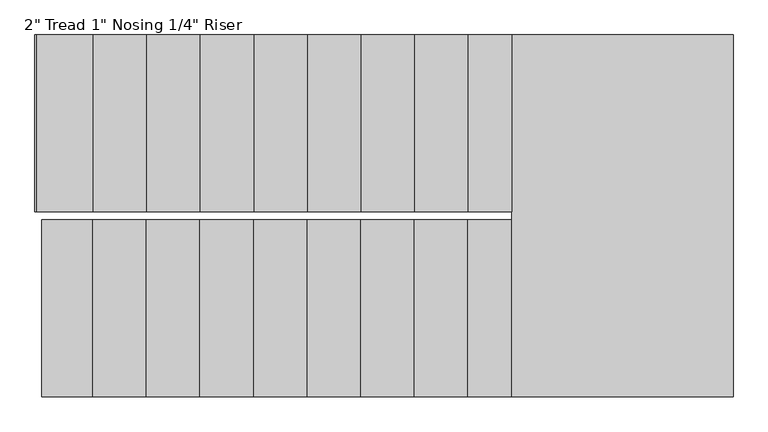
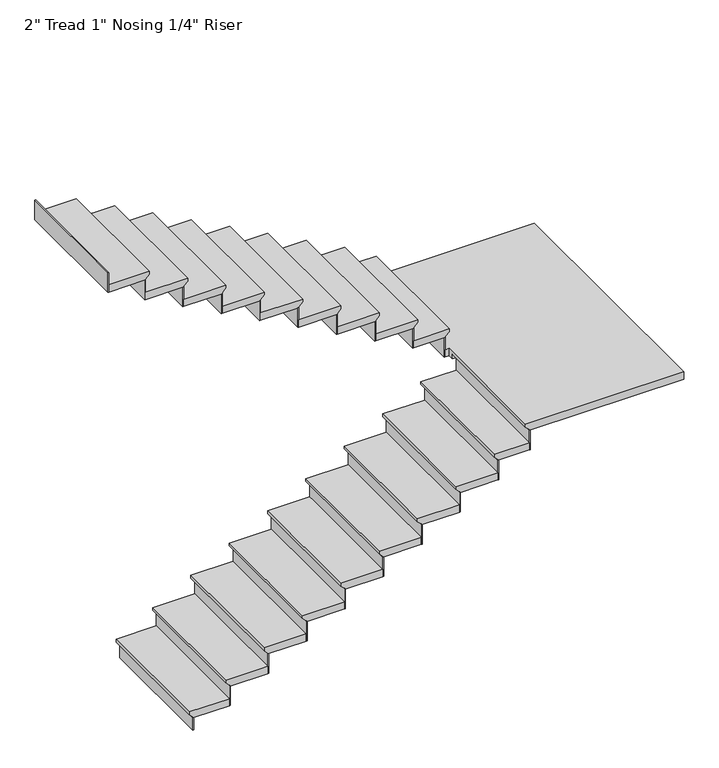
"""IFC4 building model written with IfcOpenShell, lengths in millimetres: stair flight geometry."""

from ifc_helpers import new_model, si_unit, origin, place, context, project, spatial, faceted_brep, source, transform, mapped, element, save


def stair_flight_f099b86a(model_context):
    return source(origin(), model_context, "Body", "Brep", [
        faceted_brep([(-1903.1876145, -1606.0595056, 9262.11), (-1903.1876145, -1606.0595056, 9281.16), (-1903.1876145, -767.8595056, 9281.16), (-1903.1876145, -767.8595056, 9262.11), (-1877.7876145, -1606.0595056, 9236.71), (-1877.7876145, -767.8595056, 9236.71), (-1635.543606, -1606.0595056, 9281.16), (-1635.543606, -767.8595056, 9281.16), (-1877.7876145, -767.8595056, 9230.36), (-1635.543606, -767.8595056, 9230.36), (-1635.543606, -1606.0595056, 9230.36), (-1877.7876145, -1606.0595056, 9230.36)], [[[0, 1, 2, 3]], [[4, 0, 3, 5]], [[2, 1, 6, 7]], [[8, 9, 10, 11]], [[2, 7, 9, 8, 5, 3]], [[8, 11, 4, 5]], [[6, 1, 0, 4, 11, 10]], [[7, 6, 10, 9]]]),
        faceted_brep([(-1877.7876145, -1606.0595056, 9230.36), (-1877.7876145, -1606.0595056, 9144.0), (-1871.4376145, -1606.0595056, 9144.0), (-1871.4376145, -1606.0595056, 9230.36), (-1877.7876145, -767.8595056, 9230.36), (-1871.4376145, -767.8595056, 9230.36), (-1871.4376145, -767.8595056, 9144.0), (-1877.7876145, -767.8595056, 9144.0)], [[[0, 1, 2, 3]], [[4, 5, 6, 7]], [[1, 0, 4, 7]], [[2, 1, 7, 6]], [[3, 2, 6, 5]], [[0, 3, 5, 4]]]),
        faceted_brep([(-1635.543606, -1606.0595056, 9367.52), (-1635.543606, -1606.0595056, 9230.36), (-1629.193606, -1606.0595056, 9230.36), (-1629.193606, -1606.0595056, 9367.52), (-1635.543606, -767.8595056, 9367.52), (-1629.193606, -767.8595056, 9367.52), (-1629.193606, -767.8595056, 9230.36), (-1635.543606, -767.8595056, 9230.36)], [[[0, 1, 2, 3]], [[4, 5, 6, 7]], [[1, 0, 4, 7]], [[2, 1, 7, 6]], [[3, 2, 6, 5]], [[0, 3, 5, 4]]]),
        faceted_brep([(-1660.943606, -767.8595056, 9418.32), (-1660.943606, -1606.0595056, 9418.32), (-1381.543606, -1606.0595056, 9418.32), (-1381.543606, -767.8595056, 9418.32), (-1635.543606, -767.8595056, 9367.52), (-1381.543606, -767.8595056, 9367.52), (-1381.543606, -1606.0595056, 9367.52), (-1635.543606, -1606.0595056, 9367.52), (-1635.543606, -767.8595056, 9373.87), (-1660.943606, -767.8595056, 9399.27), (-1635.543606, -1606.0595056, 9373.87), (-1660.943606, -1606.0595056, 9399.27)], [[[0, 1, 2, 3]], [[4, 5, 6, 7]], [[0, 3, 5, 4, 8, 9]], [[4, 7, 10, 8]], [[2, 1, 11, 10, 7, 6]], [[3, 2, 6, 5]], [[11, 1, 0, 9]], [[10, 11, 9, 8]]]),
        faceted_brep([(-1381.543606, -1606.0595056, 9504.68), (-1381.543606, -1606.0595056, 9367.52), (-1375.193606, -1606.0595056, 9367.52), (-1375.193606, -1606.0595056, 9504.68), (-1381.543606, -767.8595056, 9504.68), (-1375.193606, -767.8595056, 9504.68), (-1375.193606, -767.8595056, 9367.52), (-1381.543606, -767.8595056, 9367.52)], [[[0, 1, 2, 3]], [[4, 5, 6, 7]], [[1, 0, 4, 7]], [[2, 1, 7, 6]], [[3, 2, 6, 5]], [[0, 3, 5, 4]]]),
        faceted_brep([(-1406.943606, -767.8595056, 9555.48), (-1406.943606, -1606.0595056, 9555.48), (-1127.543606, -1606.0595056, 9555.48), (-1127.543606, -767.8595056, 9555.48), (-1381.543606, -767.8595056, 9504.68), (-1127.543606, -767.8595056, 9504.68), (-1127.543606, -1606.0595056, 9504.68), (-1381.543606, -1606.0595056, 9504.68), (-1381.543606, -767.8595056, 9511.03), (-1406.943606, -767.8595056, 9536.43), (-1381.543606, -1606.0595056, 9511.03), (-1406.943606, -1606.0595056, 9536.43)], [[[0, 1, 2, 3]], [[4, 5, 6, 7]], [[0, 3, 5, 4, 8, 9]], [[4, 7, 10, 8]], [[2, 1, 11, 10, 7, 6]], [[3, 2, 6, 5]], [[11, 1, 0, 9]], [[10, 11, 9, 8]]]),
        faceted_brep([(-1127.543606, -1606.0595056, 9641.84), (-1127.543606, -1606.0595056, 9504.68), (-1121.193606, -1606.0595056, 9504.68), (-1121.193606, -1606.0595056, 9641.84), (-1127.543606, -767.8595056, 9641.84), (-1121.193606, -767.8595056, 9641.84), (-1121.193606, -767.8595056, 9504.68), (-1127.543606, -767.8595056, 9504.68)], [[[0, 1, 2, 3]], [[4, 5, 6, 7]], [[1, 0, 4, 7]], [[2, 1, 7, 6]], [[3, 2, 6, 5]], [[0, 3, 5, 4]]]),
        faceted_brep([(-1152.943606, -767.8595056, 9692.64), (-1152.943606, -1606.0595056, 9692.64), (-873.543606, -1606.0595056, 9692.64), (-873.543606, -767.8595056, 9692.64), (-1127.543606, -767.8595056, 9641.84), (-873.543606, -767.8595056, 9641.84), (-873.543606, -1606.0595056, 9641.84), (-1127.543606, -1606.0595056, 9641.84), (-1127.543606, -767.8595056, 9648.19), (-1152.943606, -767.8595056, 9673.59), (-1127.543606, -1606.0595056, 9648.19), (-1152.943606, -1606.0595056, 9673.59)], [[[0, 1, 2, 3]], [[4, 5, 6, 7]], [[0, 3, 5, 4, 8, 9]], [[4, 7, 10, 8]], [[2, 1, 11, 10, 7, 6]], [[3, 2, 6, 5]], [[11, 1, 0, 9]], [[10, 11, 9, 8]]]),
        faceted_brep([(-873.543606, -1606.0595056, 9779.0), (-873.543606, -1606.0595056, 9641.84), (-867.193606, -1606.0595056, 9641.84), (-867.193606, -1606.0595056, 9779.0), (-873.543606, -767.8595056, 9779.0), (-867.193606, -767.8595056, 9779.0), (-867.193606, -767.8595056, 9641.84), (-873.543606, -767.8595056, 9641.84)], [[[0, 1, 2, 3]], [[4, 5, 6, 7]], [[1, 0, 4, 7]], [[2, 1, 7, 6]], [[3, 2, 6, 5]], [[0, 3, 5, 4]]]),
        faceted_brep([(-898.943606, -767.8595056, 9829.8), (-898.943606, -1606.0595056, 9829.8), (-619.543606, -1606.0595056, 9829.8), (-619.543606, -767.8595056, 9829.8), (-873.543606, -767.8595056, 9779.0), (-619.543606, -767.8595056, 9779.0), (-619.543606, -1606.0595056, 9779.0), (-873.543606, -1606.0595056, 9779.0), (-873.543606, -767.8595056, 9785.35), (-898.943606, -767.8595056, 9810.75), (-873.543606, -1606.0595056, 9785.35), (-898.943606, -1606.0595056, 9810.75)], [[[0, 1, 2, 3]], [[4, 5, 6, 7]], [[0, 3, 5, 4, 8, 9]], [[4, 7, 10, 8]], [[2, 1, 11, 10, 7, 6]], [[3, 2, 6, 5]], [[11, 1, 0, 9]], [[10, 11, 9, 8]]]),
        faceted_brep([(-619.543606, -1606.0595056, 9916.16), (-619.543606, -1606.0595056, 9779.0), (-613.193606, -1606.0595056, 9779.0), (-613.193606, -1606.0595056, 9916.16), (-619.543606, -767.8595056, 9916.16), (-613.193606, -767.8595056, 9916.16), (-613.193606, -767.8595056, 9779.0), (-619.543606, -767.8595056, 9779.0)], [[[0, 1, 2, 3]], [[4, 5, 6, 7]], [[1, 0, 4, 7]], [[2, 1, 7, 6]], [[3, 2, 6, 5]], [[0, 3, 5, 4]]]),
        faceted_brep([(-644.943606, -767.8595056, 9966.96), (-644.943606, -1606.0595056, 9966.96), (-365.543606, -1606.0595056, 9966.96), (-365.543606, -767.8595056, 9966.96), (-619.543606, -767.8595056, 9916.16), (-365.543606, -767.8595056, 9916.16), (-365.543606, -1606.0595056, 9916.16), (-619.543606, -1606.0595056, 9916.16), (-619.543606, -767.8595056, 9922.51), (-644.943606, -767.8595056, 9947.91), (-619.543606, -1606.0595056, 9922.51), (-644.943606, -1606.0595056, 9947.91)], [[[0, 1, 2, 3]], [[4, 5, 6, 7]], [[0, 3, 5, 4, 8, 9]], [[4, 7, 10, 8]], [[2, 1, 11, 10, 7, 6]], [[3, 2, 6, 5]], [[11, 1, 0, 9]], [[10, 11, 9, 8]]]),
        faceted_brep([(-365.543606, -1606.0595056, 10053.32), (-365.543606, -1606.0595056, 9916.16), (-359.193606, -1606.0595056, 9916.16), (-359.193606, -1606.0595056, 10053.32), (-365.543606, -767.8595056, 10053.32), (-359.193606, -767.8595056, 10053.32), (-359.193606, -767.8595056, 9916.16), (-365.543606, -767.8595056, 9916.16)], [[[0, 1, 2, 3]], [[4, 5, 6, 7]], [[1, 0, 4, 7]], [[2, 1, 7, 6]], [[3, 2, 6, 5]], [[0, 3, 5, 4]]]),
        faceted_brep([(-390.943606, -767.8595056, 10104.12), (-390.943606, -1606.0595056, 10104.12), (-111.543606, -1606.0595056, 10104.12), (-111.543606, -767.8595056, 10104.12), (-365.543606, -767.8595056, 10053.32), (-111.543606, -767.8595056, 10053.32), (-111.543606, -1606.0595056, 10053.32), (-365.543606, -1606.0595056, 10053.32), (-365.543606, -767.8595056, 10059.67), (-390.943606, -767.8595056, 10085.07), (-365.543606, -1606.0595056, 10059.67), (-390.943606, -1606.0595056, 10085.07)], [[[0, 1, 2, 3]], [[4, 5, 6, 7]], [[0, 3, 5, 4, 8, 9]], [[4, 7, 10, 8]], [[2, 1, 11, 10, 7, 6]], [[3, 2, 6, 5]], [[11, 1, 0, 9]], [[10, 11, 9, 8]]]),
        faceted_brep([(-111.543606, -1606.0595056, 10190.48), (-111.543606, -1606.0595056, 10053.32), (-105.193606, -1606.0595056, 10053.32), (-105.193606, -1606.0595056, 10190.48), (-111.543606, -767.8595056, 10190.48), (-105.193606, -767.8595056, 10190.48), (-105.193606, -767.8595056, 10053.32), (-111.543606, -767.8595056, 10053.32)], [[[0, 1, 2, 3]], [[4, 5, 6, 7]], [[1, 0, 4, 7]], [[2, 1, 7, 6]], [[3, 2, 6, 5]], [[0, 3, 5, 4]]]),
        faceted_brep([(-136.943606, -767.8595056, 10241.28), (-136.943606, -1606.0595056, 10241.28), (142.456394, -1606.0595056, 10241.28), (142.456394, -767.8595056, 10241.28), (-111.543606, -767.8595056, 10190.48), (142.456394, -767.8595056, 10190.48), (142.456394, -1606.0595056, 10190.48), (-111.543606, -1606.0595056, 10190.48), (-111.543606, -767.8595056, 10196.83), (-136.943606, -767.8595056, 10222.23), (-111.543606, -1606.0595056, 10196.83), (-136.943606, -1606.0595056, 10222.23)], [[[0, 1, 2, 3]], [[4, 5, 6, 7]], [[0, 3, 5, 4, 8, 9]], [[4, 7, 10, 8]], [[2, 1, 11, 10, 7, 6]], [[3, 2, 6, 5]], [[11, 1, 0, 9]], [[10, 11, 9, 8]]]),
        faceted_brep([(142.456394, -1606.0595056, 10327.64), (142.456394, -1606.0595056, 10190.48), (148.806394, -1606.0595056, 10190.48), (148.806394, -1606.0595056, 10327.64), (142.456394, -767.8595056, 10327.64), (148.806394, -767.8595056, 10327.64), (148.806394, -767.8595056, 10190.48), (142.456394, -767.8595056, 10190.48)], [[[0, 1, 2, 3]], [[4, 5, 6, 7]], [[1, 0, 4, 7]], [[2, 1, 7, 6]], [[3, 2, 6, 5]], [[0, 3, 5, 4]]]),
        faceted_brep([(117.056394, -767.8595056, 10378.44), (117.056394, -1606.0595056, 10378.44), (350.8830625, -1606.0595056, 10378.44), (350.8830625, -767.8595056, 10378.44), (142.456394, -767.8595056, 10327.64), (350.8830625, -767.8595056, 10327.64), (350.8830625, -1606.0595056, 10327.64), (142.456394, -1606.0595056, 10327.64), (142.456394, -767.8595056, 10333.99), (117.056394, -767.8595056, 10359.39), (142.456394, -1606.0595056, 10333.99), (117.056394, -1606.0595056, 10359.39)], [[[0, 1, 2, 3]], [[4, 5, 6, 7]], [[0, 3, 5, 4, 8, 9]], [[4, 7, 10, 8]], [[2, 1, 11, 10, 7, 6]], [[3, 2, 6, 5]], [[11, 1, 0, 9]], [[10, 11, 9, 8]]]),
        faceted_brep([(350.8830625, -1606.0595056, 10464.8), (350.8830625, -1606.0595056, 10327.64), (357.2330625, -1606.0595056, 10327.64), (357.2330625, -1606.0595056, 10464.8), (350.8830625, -767.8595056, 10464.8), (357.2330625, -767.8595056, 10464.8), (357.2330625, -767.8595056, 10327.64), (350.8830625, -767.8595056, 10327.64)], [[[0, 1, 2, 3]], [[4, 5, 6, 7]], [[1, 0, 4, 7]], [[2, 1, 7, 6]], [[3, 2, 6, 5]], [[0, 3, 5, 4]]]),
        faceted_brep([(300.0830625, -729.7595056, 10515.6), (325.4830625, -729.7595056, 10515.6), (325.4830625, -1606.0595056, 10515.6), (1373.4123855, -1606.0595056, 10515.6), (1373.4123855, 108.4404944, 10515.6), (300.0830625, 108.4404944, 10515.6), (325.4830625, -729.7595056, 10464.8), (300.0830625, -729.7595056, 10464.8), (300.0830625, 108.4404944, 10464.8), (1373.4123855, 108.4404944, 10464.8), (1373.4123855, -1606.0595056, 10464.8), (350.8830625, -1606.0595056, 10464.8), (350.8830625, -767.8595056, 10464.8), (325.4830625, -767.8595056, 10464.8), (325.4830625, -767.8595056, 10496.55), (325.4830625, -1606.0595056, 10496.55), (350.8830625, -767.8595056, 10471.15), (350.8830625, -1606.0595056, 10471.15)], [[[0, 1, 2, 3, 4, 5]], [[6, 7, 8, 9, 10, 11, 12, 13]], [[1, 0, 7, 6]], [[2, 1, 6, 13, 14, 15]], [[13, 12, 16, 14]], [[12, 11, 17, 16]], [[3, 2, 15, 17, 11, 10]], [[4, 3, 10, 9]], [[5, 4, 9, 8]], [[0, 5, 8, 7]], [[17, 15, 14, 16]]]),
        faceted_brep([(300.0830625, 108.4404944, 10601.96), (300.0830625, 108.4404944, 10464.8), (293.7330625, 108.4404944, 10464.8), (293.7330625, 108.4404944, 10601.96), (300.0830625, -729.7595056, 10601.96), (293.7330625, -729.7595056, 10601.96), (293.7330625, -729.7595056, 10464.8), (300.0830625, -729.7595056, 10464.8)], [[[0, 1, 2, 3]], [[4, 5, 6, 7]], [[1, 0, 4, 7]], [[2, 1, 7, 6]], [[3, 2, 6, 5]], [[0, 3, 5, 4]]]),
        faceted_brep([(325.4830625, -729.7595056, 10652.76), (325.4830625, 108.4404944, 10652.76), (91.656394, 108.4404944, 10652.76), (91.656394, -729.7595056, 10652.76), (300.0830625, -729.7595056, 10601.96), (91.656394, -729.7595056, 10601.96), (91.656394, 108.4404944, 10601.96), (300.0830625, 108.4404944, 10601.96), (300.0830625, -729.7595056, 10608.31), (325.4830625, -729.7595056, 10633.71), (300.0830625, 108.4404944, 10608.31), (325.4830625, 108.4404944, 10633.71)], [[[0, 1, 2, 3]], [[4, 5, 6, 7]], [[0, 3, 5, 4, 8, 9]], [[4, 7, 10, 8]], [[2, 1, 11, 10, 7, 6]], [[3, 2, 6, 5]], [[11, 1, 0, 9]], [[10, 11, 9, 8]]]),
        faceted_brep([(91.656394, 108.4404944, 10739.12), (91.656394, 108.4404944, 10601.96), (85.306394, 108.4404944, 10601.96), (85.306394, 108.4404944, 10739.12), (91.656394, -729.7595056, 10739.12), (85.306394, -729.7595056, 10739.12), (85.306394, -729.7595056, 10601.96), (91.656394, -729.7595056, 10601.96)], [[[0, 1, 2, 3]], [[4, 5, 6, 7]], [[1, 0, 4, 7]], [[2, 1, 7, 6]], [[3, 2, 6, 5]], [[0, 3, 5, 4]]]),
        faceted_brep([(117.056394, -729.7595056, 10789.92), (117.056394, 108.4404944, 10789.92), (-162.343606, 108.4404944, 10789.92), (-162.343606, -729.7595056, 10789.92), (91.656394, -729.7595056, 10739.12), (-162.343606, -729.7595056, 10739.12), (-162.343606, 108.4404944, 10739.12), (91.656394, 108.4404944, 10739.12), (91.656394, -729.7595056, 10745.47), (117.056394, -729.7595056, 10770.87), (91.656394, 108.4404944, 10745.47), (117.056394, 108.4404944, 10770.87)], [[[0, 1, 2, 3]], [[4, 5, 6, 7]], [[0, 3, 5, 4, 8, 9]], [[4, 7, 10, 8]], [[2, 1, 11, 10, 7, 6]], [[3, 2, 6, 5]], [[11, 1, 0, 9]], [[10, 11, 9, 8]]]),
        faceted_brep([(-162.343606, 108.4404944, 10876.28), (-162.343606, 108.4404944, 10739.12), (-168.693606, 108.4404944, 10739.12), (-168.693606, 108.4404944, 10876.28), (-162.343606, -729.7595056, 10876.28), (-168.693606, -729.7595056, 10876.28), (-168.693606, -729.7595056, 10739.12), (-162.343606, -729.7595056, 10739.12)], [[[0, 1, 2, 3]], [[4, 5, 6, 7]], [[1, 0, 4, 7]], [[2, 1, 7, 6]], [[3, 2, 6, 5]], [[0, 3, 5, 4]]]),
        faceted_brep([(-136.943606, -729.7595056, 10927.08), (-136.943606, 108.4404944, 10927.08), (-416.343606, 108.4404944, 10927.08), (-416.343606, -729.7595056, 10927.08), (-162.343606, -729.7595056, 10876.28), (-416.343606, -729.7595056, 10876.28), (-416.343606, 108.4404944, 10876.28), (-162.343606, 108.4404944, 10876.28), (-162.343606, -729.7595056, 10882.63), (-136.943606, -729.7595056, 10908.03), (-162.343606, 108.4404944, 10882.63), (-136.943606, 108.4404944, 10908.03)], [[[0, 1, 2, 3]], [[4, 5, 6, 7]], [[0, 3, 5, 4, 8, 9]], [[4, 7, 10, 8]], [[2, 1, 11, 10, 7, 6]], [[3, 2, 6, 5]], [[11, 1, 0, 9]], [[10, 11, 9, 8]]]),
        faceted_brep([(-416.343606, 108.4404944, 11013.44), (-416.343606, 108.4404944, 10876.28), (-422.693606, 108.4404944, 10876.28), (-422.693606, 108.4404944, 11013.44), (-416.343606, -729.7595056, 11013.44), (-422.693606, -729.7595056, 11013.44), (-422.693606, -729.7595056, 10876.28), (-416.343606, -729.7595056, 10876.28)], [[[0, 1, 2, 3]], [[4, 5, 6, 7]], [[1, 0, 4, 7]], [[2, 1, 7, 6]], [[3, 2, 6, 5]], [[0, 3, 5, 4]]]),
        faceted_brep([(-390.943606, -729.7595056, 11064.24), (-390.943606, 108.4404944, 11064.24), (-670.343606, 108.4404944, 11064.24), (-670.343606, -729.7595056, 11064.24), (-416.343606, -729.7595056, 11013.44), (-670.343606, -729.7595056, 11013.44), (-670.343606, 108.4404944, 11013.44), (-416.343606, 108.4404944, 11013.44), (-416.343606, -729.7595056, 11019.79), (-390.943606, -729.7595056, 11045.19), (-416.343606, 108.4404944, 11019.79), (-390.943606, 108.4404944, 11045.19)], [[[0, 1, 2, 3]], [[4, 5, 6, 7]], [[0, 3, 5, 4, 8, 9]], [[4, 7, 10, 8]], [[2, 1, 11, 10, 7, 6]], [[3, 2, 6, 5]], [[11, 1, 0, 9]], [[10, 11, 9, 8]]]),
        faceted_brep([(-670.343606, 108.4404944, 11150.6), (-670.343606, 108.4404944, 11013.44), (-676.693606, 108.4404944, 11013.44), (-676.693606, 108.4404944, 11150.6), (-670.343606, -729.7595056, 11150.6), (-676.693606, -729.7595056, 11150.6), (-676.693606, -729.7595056, 11013.44), (-670.343606, -729.7595056, 11013.44)], [[[0, 1, 2, 3]], [[4, 5, 6, 7]], [[1, 0, 4, 7]], [[2, 1, 7, 6]], [[3, 2, 6, 5]], [[0, 3, 5, 4]]]),
        faceted_brep([(-644.943606, -729.7595056, 11201.4), (-644.943606, 108.4404944, 11201.4), (-924.343606, 108.4404944, 11201.4), (-924.343606, -729.7595056, 11201.4), (-670.343606, -729.7595056, 11150.6), (-924.343606, -729.7595056, 11150.6), (-924.343606, 108.4404944, 11150.6), (-670.343606, 108.4404944, 11150.6), (-670.343606, -729.7595056, 11156.95), (-644.943606, -729.7595056, 11182.35), (-670.343606, 108.4404944, 11156.95), (-644.943606, 108.4404944, 11182.35)], [[[0, 1, 2, 3]], [[4, 5, 6, 7]], [[0, 3, 5, 4, 8, 9]], [[4, 7, 10, 8]], [[2, 1, 11, 10, 7, 6]], [[3, 2, 6, 5]], [[11, 1, 0, 9]], [[10, 11, 9, 8]]]),
        faceted_brep([(-924.343606, 108.4404944, 11287.76), (-924.343606, 108.4404944, 11150.6), (-930.693606, 108.4404944, 11150.6), (-930.693606, 108.4404944, 11287.76), (-924.343606, -729.7595056, 11287.76), (-930.693606, -729.7595056, 11287.76), (-930.693606, -729.7595056, 11150.6), (-924.343606, -729.7595056, 11150.6)], [[[0, 1, 2, 3]], [[4, 5, 6, 7]], [[1, 0, 4, 7]], [[2, 1, 7, 6]], [[3, 2, 6, 5]], [[0, 3, 5, 4]]]),
        faceted_brep([(-898.943606, -729.7595056, 11338.56), (-898.943606, 108.4404944, 11338.56), (-1178.343606, 108.4404944, 11338.56), (-1178.343606, -729.7595056, 11338.56), (-924.343606, -729.7595056, 11287.76), (-1178.343606, -729.7595056, 11287.76), (-1178.343606, 108.4404944, 11287.76), (-924.343606, 108.4404944, 11287.76), (-924.343606, -729.7595056, 11294.11), (-898.943606, -729.7595056, 11319.51), (-924.343606, 108.4404944, 11294.11), (-898.943606, 108.4404944, 11319.51)], [[[0, 1, 2, 3]], [[4, 5, 6, 7]], [[0, 3, 5, 4, 8, 9]], [[4, 7, 10, 8]], [[2, 1, 11, 10, 7, 6]], [[3, 2, 6, 5]], [[11, 1, 0, 9]], [[10, 11, 9, 8]]]),
        faceted_brep([(-1178.343606, 108.4404944, 11424.92), (-1178.343606, 108.4404944, 11287.76), (-1184.693606, 108.4404944, 11287.76), (-1184.693606, 108.4404944, 11424.92), (-1178.343606, -729.7595056, 11424.92), (-1184.693606, -729.7595056, 11424.92), (-1184.693606, -729.7595056, 11287.76), (-1178.343606, -729.7595056, 11287.76)], [[[0, 1, 2, 3]], [[4, 5, 6, 7]], [[1, 0, 4, 7]], [[2, 1, 7, 6]], [[3, 2, 6, 5]], [[0, 3, 5, 4]]]),
        faceted_brep([(-1152.943606, -729.7595056, 11475.72), (-1152.943606, 108.4404944, 11475.72), (-1432.343606, 108.4404944, 11475.72), (-1432.343606, -729.7595056, 11475.72), (-1178.343606, -729.7595056, 11424.92), (-1432.343606, -729.7595056, 11424.92), (-1432.343606, 108.4404944, 11424.92), (-1178.343606, 108.4404944, 11424.92), (-1178.343606, -729.7595056, 11431.27), (-1152.943606, -729.7595056, 11456.67), (-1178.343606, 108.4404944, 11431.27), (-1152.943606, 108.4404944, 11456.67)], [[[0, 1, 2, 3]], [[4, 5, 6, 7]], [[0, 3, 5, 4, 8, 9]], [[4, 7, 10, 8]], [[2, 1, 11, 10, 7, 6]], [[3, 2, 6, 5]], [[11, 1, 0, 9]], [[10, 11, 9, 8]]]),
        faceted_brep([(-1432.343606, 108.4404944, 11562.08), (-1432.343606, 108.4404944, 11424.92), (-1438.693606, 108.4404944, 11424.92), (-1438.693606, 108.4404944, 11562.08), (-1432.343606, -729.7595056, 11562.08), (-1438.693606, -729.7595056, 11562.08), (-1438.693606, -729.7595056, 11424.92), (-1432.343606, -729.7595056, 11424.92)], [[[0, 1, 2, 3]], [[4, 5, 6, 7]], [[1, 0, 4, 7]], [[2, 1, 7, 6]], [[3, 2, 6, 5]], [[0, 3, 5, 4]]]),
        faceted_brep([(-1406.943606, -729.7595056, 11612.88), (-1406.943606, 108.4404944, 11612.88), (-1686.343606, 108.4404944, 11612.88), (-1686.343606, -729.7595056, 11612.88), (-1432.343606, -729.7595056, 11562.08), (-1686.343606, -729.7595056, 11562.08), (-1686.343606, 108.4404944, 11562.08), (-1432.343606, 108.4404944, 11562.08), (-1432.343606, -729.7595056, 11568.43), (-1406.943606, -729.7595056, 11593.83), (-1432.343606, 108.4404944, 11568.43), (-1406.943606, 108.4404944, 11593.83)], [[[0, 1, 2, 3]], [[4, 5, 6, 7]], [[0, 3, 5, 4, 8, 9]], [[4, 7, 10, 8]], [[2, 1, 11, 10, 7, 6]], [[3, 2, 6, 5]], [[11, 1, 0, 9]], [[10, 11, 9, 8]]]),
        faceted_brep([(-1686.343606, 108.4404944, 11699.24), (-1686.343606, 108.4404944, 11562.08), (-1692.693606, 108.4404944, 11562.08), (-1692.693606, 108.4404944, 11699.24), (-1686.343606, -729.7595056, 11699.24), (-1692.693606, -729.7595056, 11699.24), (-1692.693606, -729.7595056, 11562.08), (-1686.343606, -729.7595056, 11562.08)], [[[0, 1, 2, 3]], [[4, 5, 6, 7]], [[1, 0, 4, 7]], [[2, 1, 7, 6]], [[3, 2, 6, 5]], [[0, 3, 5, 4]]]),
        faceted_brep([(-1928.5876145, 108.4404944, 11836.4), (-1928.5876145, 108.4404944, 11699.24), (-1934.9376145, 108.4404944, 11699.24), (-1934.9376145, 108.4404944, 11836.4), (-1928.5876145, -729.7595056, 11836.4), (-1934.9376145, -729.7595056, 11836.4), (-1934.9376145, -729.7595056, 11699.24), (-1928.5876145, -729.7595056, 11699.24)], [[[0, 1, 2, 3]], [[4, 5, 6, 7]], [[1, 0, 4, 7]], [[2, 1, 7, 6]], [[3, 2, 6, 5]], [[0, 3, 5, 4]]]),
        faceted_brep([(-1660.943606, -729.7595056, 11750.04), (-1660.943606, 108.4404944, 11750.04), (-1928.5876145, 108.4404944, 11750.04), (-1928.5876145, -729.7595056, 11750.04), (-1686.343606, -729.7595056, 11699.24), (-1928.5876145, -729.7595056, 11699.24), (-1928.5876145, 108.4404944, 11699.24), (-1686.343606, 108.4404944, 11699.24), (-1686.343606, -729.7595056, 11705.59), (-1660.943606, -729.7595056, 11730.99), (-1686.343606, 108.4404944, 11705.59), (-1660.943606, 108.4404944, 11730.99)], [[[0, 1, 2, 3]], [[4, 5, 6, 7]], [[0, 3, 5, 4, 8, 9]], [[4, 7, 10, 8]], [[2, 1, 11, 10, 7, 6]], [[3, 2, 6, 5]], [[11, 1, 0, 9]], [[10, 11, 9, 8]]]),
    ])


if __name__ == "__main__":
    model = new_model("IFC4")
    model_context = context("Model", 3, world=origin())
    ifc_project = project(units=[si_unit("LENGTHUNIT", "METRE", prefix="MILLI")], contexts=[model_context])
    site = spatial("IfcSite", under=ifc_project)
    building = spatial("IfcBuilding", under=site)
    placement = place(None, origin())
    stair_flight_shape = stair_flight_f099b86a(model_context)
    element("IfcStairFlight", 1, ObjectType="2\" Tread 1\" Nosing 1/4\" Riser", at=placement, inside=building, context=model_context, shape_type="MappedRepresentation", body=[
        mapped(stair_flight_shape, transform((0.0, 0.0, 0.0), x_axis=(1.0, 0.0, 0.0), y_axis=(0.0, 1.0, 0.0), z_axis=(0.0, 0.0, 1.0))),
    ])
    save(model, "model.ifc")
